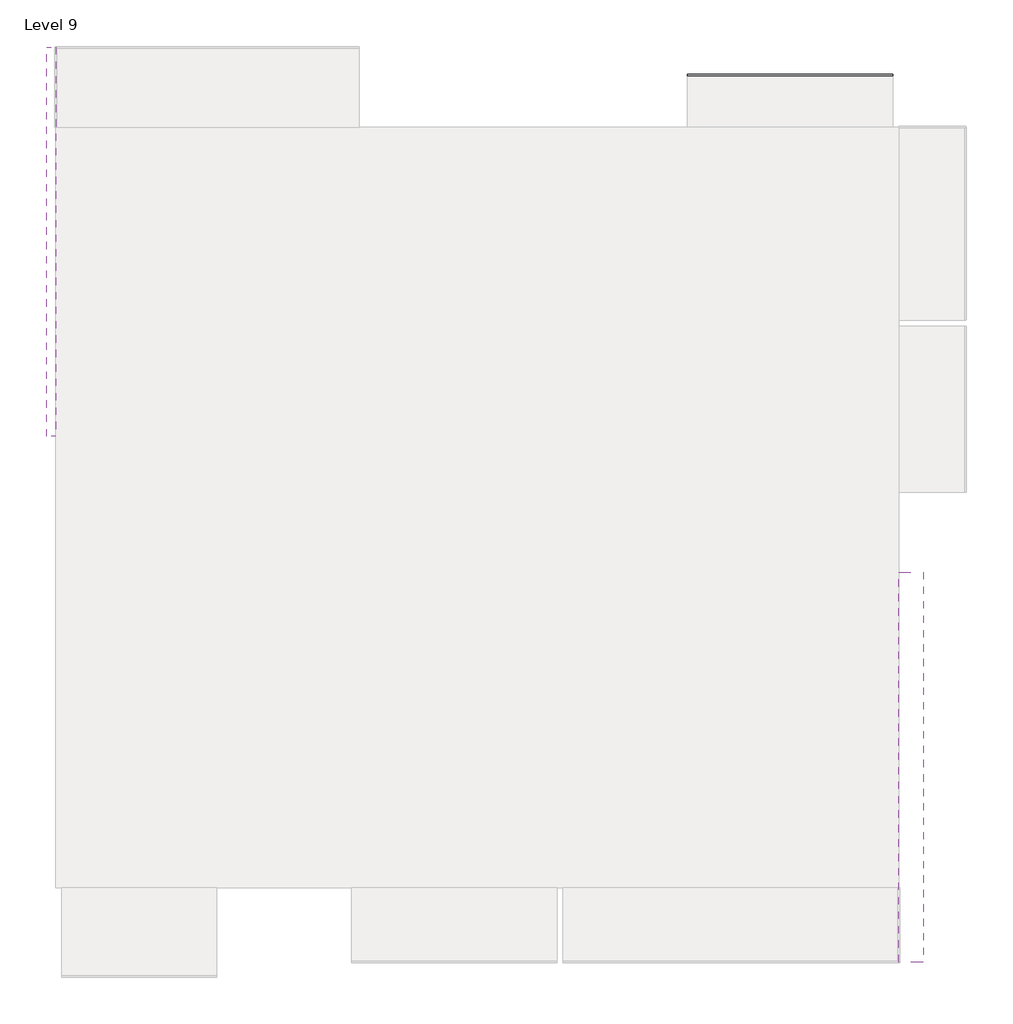
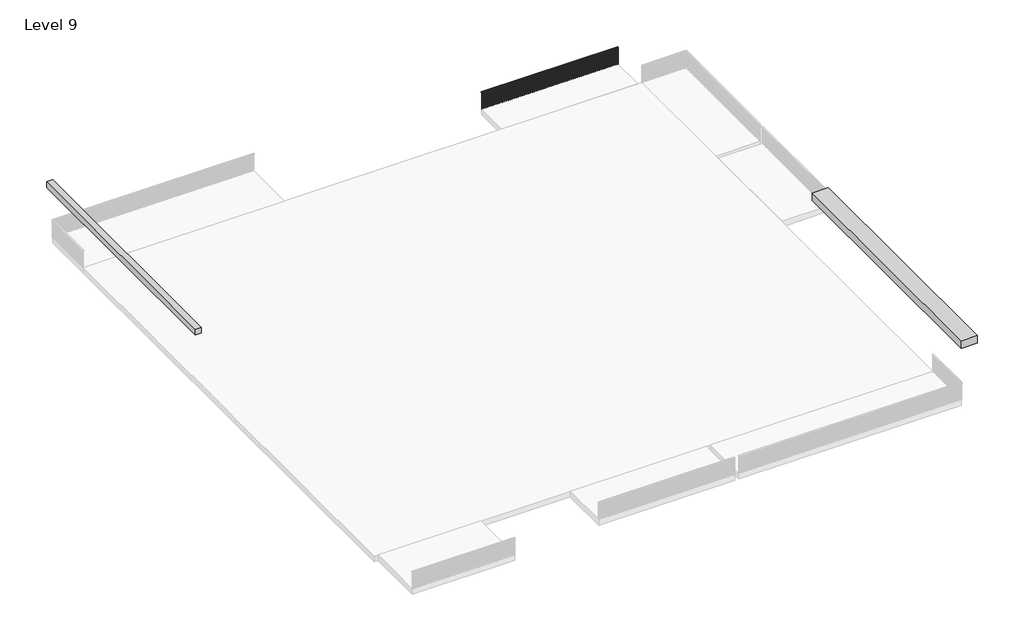
# One storey, part 5 of 5: 2 proxies, 1 railing.
"""IFC4 building model written with IfcOpenShell, lengths in millimetres."""

from ifc_helpers import new_model, si_unit, frame, origin, place, context, project, spatial, polyline, outline, extrude, transform, mapped, element, save
from components import generic_models_10_generic_models_8_4a409525, generic_models_6_generic_models_4_f66e2b9f

model = new_model("IFC4")

# Units and contexts
model_context = context("Model", 3, world=origin())
ifc_project = project(units=[si_unit("LENGTHUNIT", "METRE", prefix="MILLI")], contexts=[model_context])

# Site, building, storey
site = spatial("IfcSite", under=ifc_project)
building = spatial("IfcBuilding", under=site)
storey = spatial("IfcBuildingStorey", under=building, Name="Level 9", Elevation=9448.8)

# Proxies
placement = place(None, origin())
generic_models_10_generic_models_8_shape = generic_models_10_generic_models_8_4a409525(model_context)
element("IfcBuildingElementProxy", 1, Name="Generic Models 10 : Generic Models 8", ObjectType="Generic Models 10 : Generic Models 8", at=placement, inside=storey, context=model_context, shape_type="MappedRepresentation", body=[
    mapped(generic_models_10_generic_models_8_shape, transform((0.0, 0.0, -6248.4), x_axis=(1.0, 0.0, 0.0), y_axis=(0.0, 1.0, 0.0), z_axis=(0.0, 0.0, 1.0))),
])
generic_models_6_generic_models_4_shape = generic_models_6_generic_models_4_f66e2b9f(model_context)
element("IfcBuildingElementProxy", 2, Name="Generic Models 6 : Generic Models 4", ObjectType="Generic Models 6 : Generic Models 4", at=placement, inside=storey, context=model_context, shape_type="MappedRepresentation", body=[
    mapped(generic_models_6_generic_models_4_shape, transform((0.0, 7.836402, 6263.6678902), x_axis=(1.0, 0.0, 0.0), y_axis=(0.0, 1.0, 0.0), z_axis=(0.0, 0.0, 1.0))),
])

# Railing
element("IfcRailing", 3, ObjectType="Handrail - Rectangular", at=placement, inside=storey, context=model_context, shape_type="SweptSolid", body=[
    extrude(outline(polyline([(7096.1361222, 16470.4237525), (7096.1361222, 16521.2237525), (13903.3361222, 16521.2237525), (13903.3361222, 16470.4237525), (7096.1361222, 16470.4237525)])), frame((0.0, 0.0, 10312.4), z_axis=(0.0, 0.0, 1.0), x_axis=(1.0, 0.0, 0.0)), (0.0, 0.0, 1.0), 50.8),
    extrude(outline(polyline([(13792.2111222, 16486.2987525), (13792.2111222, 16505.3487525), (13811.2611222, 16505.3487525), (13811.2611222, 16486.2987525), (13792.2111222, 16486.2987525)])), frame((0.0, 0.0, 9448.8), z_axis=(0.0, 0.0, 1.0), x_axis=(1.0, 0.0, 0.0)), (0.0, 0.0, 1.0), 863.6),
    extrude(outline(polyline([(13690.6111222, 16486.2987525), (13690.6111222, 16505.3487525), (13709.6611222, 16505.3487525), (13709.6611222, 16486.2987525), (13690.6111222, 16486.2987525)])), frame((0.0, 0.0, 9448.8), z_axis=(0.0, 0.0, 1.0), x_axis=(1.0, 0.0, 0.0)), (0.0, 0.0, 1.0), 863.6),
    extrude(outline(polyline([(13589.0111222, 16486.2987525), (13589.0111222, 16505.3487525), (13608.0611222, 16505.3487525), (13608.0611222, 16486.2987525), (13589.0111222, 16486.2987525)])), frame((0.0, 0.0, 9448.8), z_axis=(0.0, 0.0, 1.0), x_axis=(1.0, 0.0, 0.0)), (0.0, 0.0, 1.0), 863.6),
    extrude(outline(polyline([(13487.4111222, 16486.2987525), (13487.4111222, 16505.3487525), (13506.4611222, 16505.3487525), (13506.4611222, 16486.2987525), (13487.4111222, 16486.2987525)])), frame((0.0, 0.0, 9448.8), z_axis=(0.0, 0.0, 1.0), x_axis=(1.0, 0.0, 0.0)), (0.0, 0.0, 1.0), 863.6),
    extrude(outline(polyline([(13385.8111222, 16486.2987525), (13385.8111222, 16505.3487525), (13404.8611222, 16505.3487525), (13404.8611222, 16486.2987525), (13385.8111222, 16486.2987525)])), frame((0.0, 0.0, 9448.8), z_axis=(0.0, 0.0, 1.0), x_axis=(1.0, 0.0, 0.0)), (0.0, 0.0, 1.0), 863.6),
    extrude(outline(polyline([(13284.2111222, 16486.2987525), (13284.2111222, 16505.3487525), (13303.2611222, 16505.3487525), (13303.2611222, 16486.2987525), (13284.2111222, 16486.2987525)])), frame((0.0, 0.0, 9448.8), z_axis=(0.0, 0.0, 1.0), x_axis=(1.0, 0.0, 0.0)), (0.0, 0.0, 1.0), 863.6),
    extrude(outline(polyline([(13182.6111222, 16486.2987525), (13182.6111222, 16505.3487525), (13201.6611222, 16505.3487525), (13201.6611222, 16486.2987525), (13182.6111222, 16486.2987525)])), frame((0.0, 0.0, 9448.8), z_axis=(0.0, 0.0, 1.0), x_axis=(1.0, 0.0, 0.0)), (0.0, 0.0, 1.0), 863.6),
    extrude(outline(polyline([(13081.0111222, 16486.2987525), (13081.0111222, 16505.3487525), (13100.0611222, 16505.3487525), (13100.0611222, 16486.2987525), (13081.0111222, 16486.2987525)])), frame((0.0, 0.0, 9448.8), z_axis=(0.0, 0.0, 1.0), x_axis=(1.0, 0.0, 0.0)), (0.0, 0.0, 1.0), 863.6),
    extrude(outline(polyline([(12979.4111222, 16486.2987525), (12979.4111222, 16505.3487525), (12998.4611222, 16505.3487525), (12998.4611222, 16486.2987525), (12979.4111222, 16486.2987525)])), frame((0.0, 0.0, 9448.8), z_axis=(0.0, 0.0, 1.0), x_axis=(1.0, 0.0, 0.0)), (0.0, 0.0, 1.0), 863.6),
    extrude(outline(polyline([(12877.8111222, 16486.2987525), (12877.8111222, 16505.3487525), (12896.8611222, 16505.3487525), (12896.8611222, 16486.2987525), (12877.8111222, 16486.2987525)])), frame((0.0, 0.0, 9448.8), z_axis=(0.0, 0.0, 1.0), x_axis=(1.0, 0.0, 0.0)), (0.0, 0.0, 1.0), 863.6),
    extrude(outline(polyline([(12776.2111222, 16486.2987525), (12776.2111222, 16505.3487525), (12795.2611222, 16505.3487525), (12795.2611222, 16486.2987525), (12776.2111222, 16486.2987525)])), frame((0.0, 0.0, 9448.8), z_axis=(0.0, 0.0, 1.0), x_axis=(1.0, 0.0, 0.0)), (0.0, 0.0, 1.0), 863.6),
    extrude(outline(polyline([(12674.6111222, 16486.2987525), (12674.6111222, 16505.3487525), (12693.6611222, 16505.3487525), (12693.6611222, 16486.2987525), (12674.6111222, 16486.2987525)])), frame((0.0, 0.0, 9448.8), z_axis=(0.0, 0.0, 1.0), x_axis=(1.0, 0.0, 0.0)), (0.0, 0.0, 1.0), 863.6),
    extrude(outline(polyline([(12573.0111222, 16486.2987525), (12573.0111222, 16505.3487525), (12592.0611222, 16505.3487525), (12592.0611222, 16486.2987525), (12573.0111222, 16486.2987525)])), frame((0.0, 0.0, 9448.8), z_axis=(0.0, 0.0, 1.0), x_axis=(1.0, 0.0, 0.0)), (0.0, 0.0, 1.0), 863.6),
    extrude(outline(polyline([(12471.4111222, 16486.2987525), (12471.4111222, 16505.3487525), (12490.4611222, 16505.3487525), (12490.4611222, 16486.2987525), (12471.4111222, 16486.2987525)])), frame((0.0, 0.0, 9448.8), z_axis=(0.0, 0.0, 1.0), x_axis=(1.0, 0.0, 0.0)), (0.0, 0.0, 1.0), 863.6),
    extrude(outline(polyline([(12369.8111222, 16486.2987525), (12369.8111222, 16505.3487525), (12388.8611222, 16505.3487525), (12388.8611222, 16486.2987525), (12369.8111222, 16486.2987525)])), frame((0.0, 0.0, 9448.8), z_axis=(0.0, 0.0, 1.0), x_axis=(1.0, 0.0, 0.0)), (0.0, 0.0, 1.0), 863.6),
    extrude(outline(polyline([(12268.2111222, 16486.2987525), (12268.2111222, 16505.3487525), (12287.2611222, 16505.3487525), (12287.2611222, 16486.2987525), (12268.2111222, 16486.2987525)])), frame((0.0, 0.0, 9448.8), z_axis=(0.0, 0.0, 1.0), x_axis=(1.0, 0.0, 0.0)), (0.0, 0.0, 1.0), 863.6),
    extrude(outline(polyline([(12166.6111222, 16486.2987525), (12166.6111222, 16505.3487525), (12185.6611222, 16505.3487525), (12185.6611222, 16486.2987525), (12166.6111222, 16486.2987525)])), frame((0.0, 0.0, 9448.8), z_axis=(0.0, 0.0, 1.0), x_axis=(1.0, 0.0, 0.0)), (0.0, 0.0, 1.0), 863.6),
    extrude(outline(polyline([(12065.0111222, 16486.2987525), (12065.0111222, 16505.3487525), (12084.0611222, 16505.3487525), (12084.0611222, 16486.2987525), (12065.0111222, 16486.2987525)])), frame((0.0, 0.0, 9448.8), z_axis=(0.0, 0.0, 1.0), x_axis=(1.0, 0.0, 0.0)), (0.0, 0.0, 1.0), 863.6),
    extrude(outline(polyline([(11963.4111222, 16486.2987525), (11963.4111222, 16505.3487525), (11982.4611222, 16505.3487525), (11982.4611222, 16486.2987525), (11963.4111222, 16486.2987525)])), frame((0.0, 0.0, 9448.8), z_axis=(0.0, 0.0, 1.0), x_axis=(1.0, 0.0, 0.0)), (0.0, 0.0, 1.0), 863.6),
    extrude(outline(polyline([(11861.8111222, 16486.2987525), (11861.8111222, 16505.3487525), (11880.8611222, 16505.3487525), (11880.8611222, 16486.2987525), (11861.8111222, 16486.2987525)])), frame((0.0, 0.0, 9448.8), z_axis=(0.0, 0.0, 1.0), x_axis=(1.0, 0.0, 0.0)), (0.0, 0.0, 1.0), 863.6),
    extrude(outline(polyline([(11760.2111222, 16486.2987525), (11760.2111222, 16505.3487525), (11779.2611222, 16505.3487525), (11779.2611222, 16486.2987525), (11760.2111222, 16486.2987525)])), frame((0.0, 0.0, 9448.8), z_axis=(0.0, 0.0, 1.0), x_axis=(1.0, 0.0, 0.0)), (0.0, 0.0, 1.0), 863.6),
    extrude(outline(polyline([(11658.6111222, 16486.2987525), (11658.6111222, 16505.3487525), (11677.6611222, 16505.3487525), (11677.6611222, 16486.2987525), (11658.6111222, 16486.2987525)])), frame((0.0, 0.0, 9448.8), z_axis=(0.0, 0.0, 1.0), x_axis=(1.0, 0.0, 0.0)), (0.0, 0.0, 1.0), 863.6),
    extrude(outline(polyline([(11557.0111222, 16486.2987525), (11557.0111222, 16505.3487525), (11576.0611222, 16505.3487525), (11576.0611222, 16486.2987525), (11557.0111222, 16486.2987525)])), frame((0.0, 0.0, 9448.8), z_axis=(0.0, 0.0, 1.0), x_axis=(1.0, 0.0, 0.0)), (0.0, 0.0, 1.0), 863.6),
    extrude(outline(polyline([(11455.4111222, 16486.2987525), (11455.4111222, 16505.3487525), (11474.4611222, 16505.3487525), (11474.4611222, 16486.2987525), (11455.4111222, 16486.2987525)])), frame((0.0, 0.0, 9448.8), z_axis=(0.0, 0.0, 1.0), x_axis=(1.0, 0.0, 0.0)), (0.0, 0.0, 1.0), 863.6),
    extrude(outline(polyline([(11353.8111222, 16486.2987525), (11353.8111222, 16505.3487525), (11372.8611222, 16505.3487525), (11372.8611222, 16486.2987525), (11353.8111222, 16486.2987525)])), frame((0.0, 0.0, 9448.8), z_axis=(0.0, 0.0, 1.0), x_axis=(1.0, 0.0, 0.0)), (0.0, 0.0, 1.0), 863.6),
    extrude(outline(polyline([(11252.2111222, 16486.2987525), (11252.2111222, 16505.3487525), (11271.2611222, 16505.3487525), (11271.2611222, 16486.2987525), (11252.2111222, 16486.2987525)])), frame((0.0, 0.0, 9448.8), z_axis=(0.0, 0.0, 1.0), x_axis=(1.0, 0.0, 0.0)), (0.0, 0.0, 1.0), 863.6),
    extrude(outline(polyline([(11150.6111222, 16486.2987525), (11150.6111222, 16505.3487525), (11169.6611222, 16505.3487525), (11169.6611222, 16486.2987525), (11150.6111222, 16486.2987525)])), frame((0.0, 0.0, 9448.8), z_axis=(0.0, 0.0, 1.0), x_axis=(1.0, 0.0, 0.0)), (0.0, 0.0, 1.0), 863.6),
    extrude(outline(polyline([(11049.0111222, 16486.2987525), (11049.0111222, 16505.3487525), (11068.0611222, 16505.3487525), (11068.0611222, 16486.2987525), (11049.0111222, 16486.2987525)])), frame((0.0, 0.0, 9448.8), z_axis=(0.0, 0.0, 1.0), x_axis=(1.0, 0.0, 0.0)), (0.0, 0.0, 1.0), 863.6),
    extrude(outline(polyline([(10947.4111222, 16486.2987525), (10947.4111222, 16505.3487525), (10966.4611222, 16505.3487525), (10966.4611222, 16486.2987525), (10947.4111222, 16486.2987525)])), frame((0.0, 0.0, 9448.8), z_axis=(0.0, 0.0, 1.0), x_axis=(1.0, 0.0, 0.0)), (0.0, 0.0, 1.0), 863.6),
    extrude(outline(polyline([(10845.8111222, 16486.2987525), (10845.8111222, 16505.3487525), (10864.8611222, 16505.3487525), (10864.8611222, 16486.2987525), (10845.8111222, 16486.2987525)])), frame((0.0, 0.0, 9448.8), z_axis=(0.0, 0.0, 1.0), x_axis=(1.0, 0.0, 0.0)), (0.0, 0.0, 1.0), 863.6),
    extrude(outline(polyline([(10744.2111222, 16486.2987525), (10744.2111222, 16505.3487525), (10763.2611222, 16505.3487525), (10763.2611222, 16486.2987525), (10744.2111222, 16486.2987525)])), frame((0.0, 0.0, 9448.8), z_axis=(0.0, 0.0, 1.0), x_axis=(1.0, 0.0, 0.0)), (0.0, 0.0, 1.0), 863.6),
    extrude(outline(polyline([(10642.6111222, 16486.2987525), (10642.6111222, 16505.3487525), (10661.6611222, 16505.3487525), (10661.6611222, 16486.2987525), (10642.6111222, 16486.2987525)])), frame((0.0, 0.0, 9448.8), z_axis=(0.0, 0.0, 1.0), x_axis=(1.0, 0.0, 0.0)), (0.0, 0.0, 1.0), 863.6),
    extrude(outline(polyline([(10541.0111222, 16486.2987525), (10541.0111222, 16505.3487525), (10560.0611222, 16505.3487525), (10560.0611222, 16486.2987525), (10541.0111222, 16486.2987525)])), frame((0.0, 0.0, 9448.8), z_axis=(0.0, 0.0, 1.0), x_axis=(1.0, 0.0, 0.0)), (0.0, 0.0, 1.0), 863.6),
    extrude(outline(polyline([(10439.4111222, 16486.2987525), (10439.4111222, 16505.3487525), (10458.4611222, 16505.3487525), (10458.4611222, 16486.2987525), (10439.4111222, 16486.2987525)])), frame((0.0, 0.0, 9448.8), z_axis=(0.0, 0.0, 1.0), x_axis=(1.0, 0.0, 0.0)), (0.0, 0.0, 1.0), 863.6),
    extrude(outline(polyline([(10337.8111222, 16486.2987525), (10337.8111222, 16505.3487525), (10356.8611222, 16505.3487525), (10356.8611222, 16486.2987525), (10337.8111222, 16486.2987525)])), frame((0.0, 0.0, 9448.8), z_axis=(0.0, 0.0, 1.0), x_axis=(1.0, 0.0, 0.0)), (0.0, 0.0, 1.0), 863.6),
    extrude(outline(polyline([(10236.2111222, 16486.2987525), (10236.2111222, 16505.3487525), (10255.2611222, 16505.3487525), (10255.2611222, 16486.2987525), (10236.2111222, 16486.2987525)])), frame((0.0, 0.0, 9448.8), z_axis=(0.0, 0.0, 1.0), x_axis=(1.0, 0.0, 0.0)), (0.0, 0.0, 1.0), 863.6),
    extrude(outline(polyline([(10134.6111222, 16486.2987525), (10134.6111222, 16505.3487525), (10153.6611222, 16505.3487525), (10153.6611222, 16486.2987525), (10134.6111222, 16486.2987525)])), frame((0.0, 0.0, 9448.8), z_axis=(0.0, 0.0, 1.0), x_axis=(1.0, 0.0, 0.0)), (0.0, 0.0, 1.0), 863.6),
    extrude(outline(polyline([(10033.0111222, 16486.2987525), (10033.0111222, 16505.3487525), (10052.0611222, 16505.3487525), (10052.0611222, 16486.2987525), (10033.0111222, 16486.2987525)])), frame((0.0, 0.0, 9448.8), z_axis=(0.0, 0.0, 1.0), x_axis=(1.0, 0.0, 0.0)), (0.0, 0.0, 1.0), 863.6),
    extrude(outline(polyline([(9931.4111222, 16486.2987525), (9931.4111222, 16505.3487525), (9950.4611222, 16505.3487525), (9950.4611222, 16486.2987525), (9931.4111222, 16486.2987525)])), frame((0.0, 0.0, 9448.8), z_axis=(0.0, 0.0, 1.0), x_axis=(1.0, 0.0, 0.0)), (0.0, 0.0, 1.0), 863.6),
    extrude(outline(polyline([(9829.8111222, 16486.2987525), (9829.8111222, 16505.3487525), (9848.8611222, 16505.3487525), (9848.8611222, 16486.2987525), (9829.8111222, 16486.2987525)])), frame((0.0, 0.0, 9448.8), z_axis=(0.0, 0.0, 1.0), x_axis=(1.0, 0.0, 0.0)), (0.0, 0.0, 1.0), 863.6),
    extrude(outline(polyline([(9728.2111222, 16486.2987525), (9728.2111222, 16505.3487525), (9747.2611222, 16505.3487525), (9747.2611222, 16486.2987525), (9728.2111222, 16486.2987525)])), frame((0.0, 0.0, 9448.8), z_axis=(0.0, 0.0, 1.0), x_axis=(1.0, 0.0, 0.0)), (0.0, 0.0, 1.0), 863.6),
    extrude(outline(polyline([(9626.6111222, 16486.2987525), (9626.6111222, 16505.3487525), (9645.6611222, 16505.3487525), (9645.6611222, 16486.2987525), (9626.6111222, 16486.2987525)])), frame((0.0, 0.0, 9448.8), z_axis=(0.0, 0.0, 1.0), x_axis=(1.0, 0.0, 0.0)), (0.0, 0.0, 1.0), 863.6),
    extrude(outline(polyline([(9525.0111222, 16486.2987525), (9525.0111222, 16505.3487525), (9544.0611222, 16505.3487525), (9544.0611222, 16486.2987525), (9525.0111222, 16486.2987525)])), frame((0.0, 0.0, 9448.8), z_axis=(0.0, 0.0, 1.0), x_axis=(1.0, 0.0, 0.0)), (0.0, 0.0, 1.0), 863.6),
    extrude(outline(polyline([(9423.4111222, 16486.2987525), (9423.4111222, 16505.3487525), (9442.4611222, 16505.3487525), (9442.4611222, 16486.2987525), (9423.4111222, 16486.2987525)])), frame((0.0, 0.0, 9448.8), z_axis=(0.0, 0.0, 1.0), x_axis=(1.0, 0.0, 0.0)), (0.0, 0.0, 1.0), 863.6),
    extrude(outline(polyline([(9321.8111222, 16486.2987525), (9321.8111222, 16505.3487525), (9340.8611222, 16505.3487525), (9340.8611222, 16486.2987525), (9321.8111222, 16486.2987525)])), frame((0.0, 0.0, 9448.8), z_axis=(0.0, 0.0, 1.0), x_axis=(1.0, 0.0, 0.0)), (0.0, 0.0, 1.0), 863.6),
    extrude(outline(polyline([(9220.2111222, 16486.2987525), (9220.2111222, 16505.3487525), (9239.2611222, 16505.3487525), (9239.2611222, 16486.2987525), (9220.2111222, 16486.2987525)])), frame((0.0, 0.0, 9448.8), z_axis=(0.0, 0.0, 1.0), x_axis=(1.0, 0.0, 0.0)), (0.0, 0.0, 1.0), 863.6),
    extrude(outline(polyline([(9118.6111222, 16486.2987525), (9118.6111222, 16505.3487525), (9137.6611222, 16505.3487525), (9137.6611222, 16486.2987525), (9118.6111222, 16486.2987525)])), frame((0.0, 0.0, 9448.8), z_axis=(0.0, 0.0, 1.0), x_axis=(1.0, 0.0, 0.0)), (0.0, 0.0, 1.0), 863.6),
    extrude(outline(polyline([(9017.0111222, 16486.2987525), (9017.0111222, 16505.3487525), (9036.0611222, 16505.3487525), (9036.0611222, 16486.2987525), (9017.0111222, 16486.2987525)])), frame((0.0, 0.0, 9448.8), z_axis=(0.0, 0.0, 1.0), x_axis=(1.0, 0.0, 0.0)), (0.0, 0.0, 1.0), 863.6),
    extrude(outline(polyline([(8915.4111222, 16486.2987525), (8915.4111222, 16505.3487525), (8934.4611222, 16505.3487525), (8934.4611222, 16486.2987525), (8915.4111222, 16486.2987525)])), frame((0.0, 0.0, 9448.8), z_axis=(0.0, 0.0, 1.0), x_axis=(1.0, 0.0, 0.0)), (0.0, 0.0, 1.0), 863.6),
    extrude(outline(polyline([(8813.8111222, 16486.2987525), (8813.8111222, 16505.3487525), (8832.8611222, 16505.3487525), (8832.8611222, 16486.2987525), (8813.8111222, 16486.2987525)])), frame((0.0, 0.0, 9448.8), z_axis=(0.0, 0.0, 1.0), x_axis=(1.0, 0.0, 0.0)), (0.0, 0.0, 1.0), 863.6),
    extrude(outline(polyline([(8712.2111222, 16486.2987525), (8712.2111222, 16505.3487525), (8731.2611222, 16505.3487525), (8731.2611222, 16486.2987525), (8712.2111222, 16486.2987525)])), frame((0.0, 0.0, 9448.8), z_axis=(0.0, 0.0, 1.0), x_axis=(1.0, 0.0, 0.0)), (0.0, 0.0, 1.0), 863.6),
    extrude(outline(polyline([(8610.6111222, 16486.2987525), (8610.6111222, 16505.3487525), (8629.6611222, 16505.3487525), (8629.6611222, 16486.2987525), (8610.6111222, 16486.2987525)])), frame((0.0, 0.0, 9448.8), z_axis=(0.0, 0.0, 1.0), x_axis=(1.0, 0.0, 0.0)), (0.0, 0.0, 1.0), 863.6),
    extrude(outline(polyline([(8509.0111222, 16486.2987525), (8509.0111222, 16505.3487525), (8528.0611222, 16505.3487525), (8528.0611222, 16486.2987525), (8509.0111222, 16486.2987525)])), frame((0.0, 0.0, 9448.8), z_axis=(0.0, 0.0, 1.0), x_axis=(1.0, 0.0, 0.0)), (0.0, 0.0, 1.0), 863.6),
    extrude(outline(polyline([(8407.4111222, 16486.2987525), (8407.4111222, 16505.3487525), (8426.4611222, 16505.3487525), (8426.4611222, 16486.2987525), (8407.4111222, 16486.2987525)])), frame((0.0, 0.0, 9448.8), z_axis=(0.0, 0.0, 1.0), x_axis=(1.0, 0.0, 0.0)), (0.0, 0.0, 1.0), 863.6),
    extrude(outline(polyline([(8305.8111222, 16486.2987525), (8305.8111222, 16505.3487525), (8324.8611222, 16505.3487525), (8324.8611222, 16486.2987525), (8305.8111222, 16486.2987525)])), frame((0.0, 0.0, 9448.8), z_axis=(0.0, 0.0, 1.0), x_axis=(1.0, 0.0, 0.0)), (0.0, 0.0, 1.0), 863.6),
    extrude(outline(polyline([(8204.2111222, 16486.2987525), (8204.2111222, 16505.3487525), (8223.2611222, 16505.3487525), (8223.2611222, 16486.2987525), (8204.2111222, 16486.2987525)])), frame((0.0, 0.0, 9448.8), z_axis=(0.0, 0.0, 1.0), x_axis=(1.0, 0.0, 0.0)), (0.0, 0.0, 1.0), 863.6),
    extrude(outline(polyline([(8102.6111222, 16486.2987525), (8102.6111222, 16505.3487525), (8121.6611222, 16505.3487525), (8121.6611222, 16486.2987525), (8102.6111222, 16486.2987525)])), frame((0.0, 0.0, 9448.8), z_axis=(0.0, 0.0, 1.0), x_axis=(1.0, 0.0, 0.0)), (0.0, 0.0, 1.0), 863.6),
    extrude(outline(polyline([(8001.0111222, 16486.2987525), (8001.0111222, 16505.3487525), (8020.0611222, 16505.3487525), (8020.0611222, 16486.2987525), (8001.0111222, 16486.2987525)])), frame((0.0, 0.0, 9448.8), z_axis=(0.0, 0.0, 1.0), x_axis=(1.0, 0.0, 0.0)), (0.0, 0.0, 1.0), 863.6),
    extrude(outline(polyline([(7899.4111222, 16486.2987525), (7899.4111222, 16505.3487525), (7918.4611222, 16505.3487525), (7918.4611222, 16486.2987525), (7899.4111222, 16486.2987525)])), frame((0.0, 0.0, 9448.8), z_axis=(0.0, 0.0, 1.0), x_axis=(1.0, 0.0, 0.0)), (0.0, 0.0, 1.0), 863.6),
    extrude(outline(polyline([(7797.8111222, 16486.2987525), (7797.8111222, 16505.3487525), (7816.8611222, 16505.3487525), (7816.8611222, 16486.2987525), (7797.8111222, 16486.2987525)])), frame((0.0, 0.0, 9448.8), z_axis=(0.0, 0.0, 1.0), x_axis=(1.0, 0.0, 0.0)), (0.0, 0.0, 1.0), 863.6),
    extrude(outline(polyline([(7696.2111222, 16486.2987525), (7696.2111222, 16505.3487525), (7715.2611222, 16505.3487525), (7715.2611222, 16486.2987525), (7696.2111222, 16486.2987525)])), frame((0.0, 0.0, 9448.8), z_axis=(0.0, 0.0, 1.0), x_axis=(1.0, 0.0, 0.0)), (0.0, 0.0, 1.0), 863.6),
    extrude(outline(polyline([(7594.6111222, 16486.2987525), (7594.6111222, 16505.3487525), (7613.6611222, 16505.3487525), (7613.6611222, 16486.2987525), (7594.6111222, 16486.2987525)])), frame((0.0, 0.0, 9448.8), z_axis=(0.0, 0.0, 1.0), x_axis=(1.0, 0.0, 0.0)), (0.0, 0.0, 1.0), 863.6),
    extrude(outline(polyline([(7493.0111222, 16486.2987525), (7493.0111222, 16505.3487525), (7512.0611222, 16505.3487525), (7512.0611222, 16486.2987525), (7493.0111222, 16486.2987525)])), frame((0.0, 0.0, 9448.8), z_axis=(0.0, 0.0, 1.0), x_axis=(1.0, 0.0, 0.0)), (0.0, 0.0, 1.0), 863.6),
    extrude(outline(polyline([(7391.4111222, 16486.2987525), (7391.4111222, 16505.3487525), (7410.4611222, 16505.3487525), (7410.4611222, 16486.2987525), (7391.4111222, 16486.2987525)])), frame((0.0, 0.0, 9448.8), z_axis=(0.0, 0.0, 1.0), x_axis=(1.0, 0.0, 0.0)), (0.0, 0.0, 1.0), 863.6),
    extrude(outline(polyline([(7289.8111222, 16486.2987525), (7289.8111222, 16505.3487525), (7308.8611222, 16505.3487525), (7308.8611222, 16486.2987525), (7289.8111222, 16486.2987525)])), frame((0.0, 0.0, 9448.8), z_axis=(0.0, 0.0, 1.0), x_axis=(1.0, 0.0, 0.0)), (0.0, 0.0, 1.0), 863.6),
    extrude(outline(polyline([(7188.2111222, 16486.2987525), (7188.2111222, 16505.3487525), (7207.2611222, 16505.3487525), (7207.2611222, 16486.2987525), (7188.2111222, 16486.2987525)])), frame((0.0, 0.0, 9448.8), z_axis=(0.0, 0.0, 1.0), x_axis=(1.0, 0.0, 0.0)), (0.0, 0.0, 1.0), 863.6),
    extrude(outline(polyline([(13884.2861222, 16486.2987525), (13884.2861222, 16505.3487525), (13903.3361222, 16505.3487525), (13903.3361222, 16486.2987525), (13884.2861222, 16486.2987525)])), frame((0.0, 0.0, 9448.8), z_axis=(0.0, 0.0, 1.0), x_axis=(1.0, 0.0, 0.0)), (0.0, 0.0, 1.0), 863.6),
    extrude(outline(polyline([(7096.1361222, 16486.2987525), (7096.1361222, 16505.3487525), (7115.1861222, 16505.3487525), (7115.1861222, 16486.2987525), (7096.1361222, 16486.2987525)])), frame((0.0, 0.0, 9448.8), z_axis=(0.0, 0.0, 1.0), x_axis=(1.0, 0.0, 0.0)), (0.0, 0.0, 1.0), 863.6),
])

save(model, "model.ifc")

# Revit data of these elements
# Type "Handrail - Rectangular"
#   Assembly Code = "C2010400"
#   built-in parameter 1008612 = 0.0416667 (stored number, unit not read)
#   built-in parameter 1008611 = 0.0416667 (stored number, unit not read)
#   built-in parameter 1008609 = 0.333333 (stored number, unit not read)
#   built-in parameter 1008604 = 0.166667 (stored number, unit not read)
#   built-in parameter 1008603 = 0.166667 (stored number, unit not read)
#   Railing Height = 3' - 0"
#   built-in parameter 1008630 = 2
#   built-in parameter 1008610 = 2
#   built-in parameter 1008618 = Baluster - Square : 3/4"
# Element 1 (IfcBuildingElementProxy, "Generic Models 10 : Generic Models 8")
#   Phase Created = New Construction
# Element 2 (IfcBuildingElementProxy, "Generic Models 6 : Generic Models 4")
#   Phase Created = New Construction
# Element 3 (IfcRailing, "Handrail - Rectangular")
#   Phase Created = New Construction
